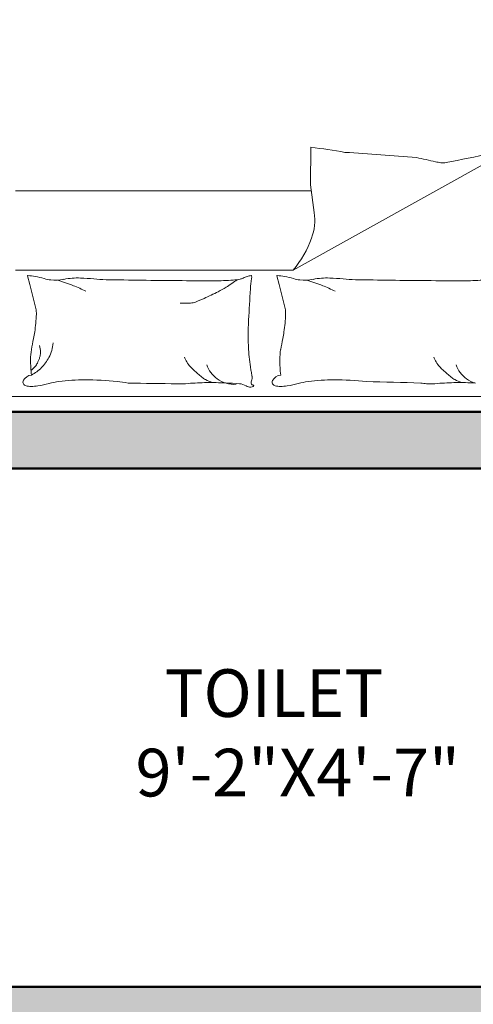
# Model space of a CAD drawing. Units: inches. Extents: x -7 to 1228, y -146 to 1091.
# Tile 72 of 88: x 674 to 722, y 785 to 890. Entities that reach past the tile are written whole.
import ezdxf

# ---------------------------------------------------------------- set-up
doc = ezdxf.new("R2010")
doc.units = ezdxf.units.IN
for name, color, linetype, lineweight in [('A-AREA-IDEN', 7, 'Continuous', 18), ('A-FURN', 8, 'Continuous', 18), ('A-WALL', 7, 'Continuous', 50), ('A-WALL-PATT', 251, 'Continuous', 13)]:
    doc.layers.add(name, color=color, linetype=linetype, lineweight=lineweight)
doc.styles.add('DIM_FONT', font='SIMPLEX.shx', dxfattribs={"width": 0.8})
doc.styles.get("Standard").update_dxf_attribs({"font": 'arial.ttf'})

# ---------------------------------------------------------------- blocks, each defined once
blk = doc.blocks.new('A$C4F634EDD')
for p, q in [((0.5, 2.6295), (2.3, 2.6295)), ((0.5, 2.5771), (2.3, 2.5771)), ((0.5953, 2.1912), (0.616, 2.2738)), ((1.4546, 2.1912), (1.4752, 2.2738)), ((0.5878, 2.1612), (0.5953, 2.1912)), ((1.4471, 2.1612), (1.4546, 2.1912)), ((1.5035, 2.141), (0.5458, 2.141)), ((1.5035, 2.141), (2.2716, 1.7136)), ((1.576, 1.9433), (1.5624, 1.8479)), ((0.5458, 1.8684), (1.5653, 1.8684)), ((1.5624, 1.8479), (1.5641, 1.7178))]:
    blk.add_line(p, q)
for centre, radius, start, end in [((0.5848, 2.5274), 0.0131, 101.2724, 206.5805), ((0.6036, 2.5368), 0.0342, 206.5805, 265.5998), ((0.5999, 2.4516), 0.0904, 90, 101.2724), ((0.5999, 2.3808), 0.1611, 81.5628, 90), ((0.5788, 2.2388), 0.3048, 74.256, 81.5628), ((0.7272, 2.7653), 0.2422, 254.256, 262.4531), ((0.7851, 3.2019), 0.6827, 262.4531, 270), ((0.7851, 3.5682), 1.049, 270, 276.0867), ((0.8402, 3.0514), 0.5293, 276.0867, 280.1899), ((1.1602, -8.1346), 10.6675, 90.30153, 91.21582), ((1.1169, 2.2433), 0.2897, 85.1982, 92.5386), ((1.2142, 3.4021), 0.8732, 265.1982, 269.4243), ((1.2362, 2.45), 0.0768, 117.2396, 128.3886), ((1.3082, 2.3102), 0.234, 110.8603, 117.2396), ((1.2204, 4.0232), 1.4943, 269.4243, 271.9079), ((1.2995, 2.4357), 0.0992, 126.0864, 143.8234), ((1.2995, 2.4357), 0.0992, 105.9352, 126.0864), ((1.2429, 3.3501), 0.8208, 271.9079, 275.2592), ((1.2995, 2.4357), 0.0992, 85.7841, 105.9352), ((1.3132, 2.5864), 0.0539, 275.2592, 300.6513), ((1.3554, 2.5152), 0.0289, 85.6975, 120.6513), ((1.3556, 2.519), 0.0251, 68.2117, 85.6975), ((1.3739, 2.5288), 0.0156, 158.0096, 201.421), ((1.3634, 2.533), 0.00428, 78.1069, 158.0096), ((1.3288, 2.5111), 0.0328, 351.8665, 21.421), ((1.3647, 2.5395), 0.00232, 258.1069, 19.564), ((1.3637, 2.5391), 0.00342, 19.564, 68.2117), ((1.444, 2.5274), 0.0131, 101.2724, 206.5805), ((1.4628, 2.5368), 0.0342, 206.5805, 265.5998), ((1.4591, 2.4516), 0.0904, 90, 101.2724), ((1.4591, 2.3808), 0.1611, 81.5628, 90), ((1.438, 2.2388), 0.3048, 74.256, 81.5628), ((1.5865, 2.7653), 0.2422, 254.256, 262.4531), ((1.6443, 3.2019), 0.6827, 262.4531, 270), ((1.6443, 3.5682), 1.049, 270, 276.0867), ((1.4785, 15.4878), 12.9656, 271.22425, 272.05324), ((1.97, 2.3805), 0.1524, 92.5386, 100.1899), ((1.9761, 2.2433), 0.2897, 85.1982, 92.5386), ((2.0734, 3.4021), 0.8732, 265.1982, 269.4243), ((2.0954, 2.45), 0.0768, 117.2396, 128.3886), ((2.1674, 2.3102), 0.234, 110.8603, 117.2396), ((2.0797, 4.0232), 1.4943, 269.4243, 271.9079), ((2.1588, 2.4357), 0.0992, 126.0864, 143.8234), ((2.1588, 2.4357), 0.0992, 105.9352, 126.0864), ((1.0898, 2.4496), 0.4918, 173.7676, 180), ((0.5462, 2.4142), 0.0899, 41.4429, 53.7359), ((0.5368, 2.3783), 0.1399, 45.0976, 62.7964), ((0.5368, 2.3783), 0.1399, 27.3988, 45.0976), ((1.3165, 2.3233), 0.2252, 133.8115, 140.9651), ((1.4317, 2.2032), 0.3916, 128.3886, 133.8115), ((1.2995, 2.4357), 0.0992, 143.8234, 161.5603), ((1.5522, 2.448), 0.1983, 167.8905, 172.3191), ((1.1177, 2.5413), 0.246, 347.8905, 351.8665), ((1.949, 2.4496), 0.4918, 173.7676, 180), ((2.1757, 2.3233), 0.2252, 133.8115, 140.9651), ((2.291, 2.2032), 0.3916, 128.3886, 133.8115), ((2.1588, 2.4357), 0.0992, 143.8234, 161.5603), ((0.8019, 2.4496), 0.204, 180, 189.6844), ((0.5741, 2.4389), 0.0526, 25.3551, 41.4429), ((0.4851, 2.3967), 0.1511, 21.8149, 25.3551), ((0.4345, 2.3765), 0.2056, 18.7799, 21.8149), ((0.576, 2.4246), 0.0562, 0, 18.7799), ((0.5368, 2.3783), 0.1399, 16.515, 27.3988), ((1.3127, 2.3625), 0.2002, 151.6832, 156.9972), ((1.1799, 2.4341), 0.0493, 140.9651, 151.6832), ((2.2605, 2.3525), 0.9131, 172.3191, 176.6313), ((1.6611, 2.4496), 0.204, 180, 189.6844), ((2.1719, 2.3625), 0.2002, 151.6832, 156.9972), ((2.0391, 2.4341), 0.0493, 140.9651, 151.6832), ((1.4703, 2.5637), 0.882, 189.6844, 192.1984), ((0.5406, 2.4246), 0.0915, 345.3149, 0), ((0.5368, 2.3783), 0.1399, 5.6311, 16.515), ((2.3295, 2.5637), 0.882, 189.6844, 192.1984), ((0.2982, 2.3103), 0.3171, 8.0051, 12.1984), ((2.0266, 2.3663), 0.6787, 176.6313, 181.6331), ((1.1575, 2.3103), 0.3171, 8.0051, 12.1984), ((-0.0401, 2.2627), 0.6588, 2.6649, 8.0051), ((2.7128, 2.3859), 1.3652, 181.6331, 183.055), ((0.8191, 2.2627), 0.6588, 2.6649, 8.0051), ((14.9657, 3.0398), 13.6356, 183.05496, 183.50486), ((0.5503, 2.2902), 0.0677, 345.9548, 2.6649), ((1.4096, 2.2902), 0.0677, 345.9548, 2.6649), ((1.1303, 1.9835), 0.2721, 85.9172, 93.5552), ((1.1455, 2.197), 0.058, 69.3257, 85.9172), ((0.9871, 1.7772), 0.5066, 65.6735, 69.3257), ((0.473, 2.8815), 0.7387, 293.4844, 295.3111), ((0.6058, 0.9338), 1.4323, 63.5015, 65.6735), ((1.1054, 1.9358), 0.3126, 57.865, 63.5015), ((1.6762, 2.2258), 0.3212, 183.5049, 189.9984), ((1.3322, 2.8815), 0.7387, 293.4844, 295.3111), ((0.6807, 2.0561), 0.1197, 96.4341, 107.3864), ((0.6836, 2.0301), 0.1459, 78.4414, 96.4341), ((0.473, 2.8815), 0.7387, 287.1982, 289.428), ((0.759, 2.3985), 0.2301, 258.4414, 272.7491), ((0.473, 2.8815), 0.7387, 289.428, 291.6577), ((0.473, 2.8815), 0.7387, 291.6577, 293.4844), ((0.7026, 3.5718), 1.4048, 272.7491, 274.6176), ((0.9136, 0.9591), 1.2165, 92.6096, 94.6176), ((1.2501, -19.8405), 22.0183, 90.37908, 91.01965), ((1.2012, -3.5404), 5.7185, 89.7135, 90.9704), ((1.224, 1.0141), 1.164, 86.426, 89.7135), ((0.8841, 1.5835), 0.7286, 54.1737, 57.865), ((1.2875, 2.0302), 0.1459, 77.131, 86.426), ((1.3099, 2.1283), 0.0453, 62.7159, 77.131), ((1.5399, 2.0561), 0.1197, 96.4341, 107.3864), ((1.5429, 2.0301), 0.1459, 78.4414, 96.4341), ((1.3322, 2.8815), 0.7387, 287.1982, 289.428), ((1.6182, 2.3985), 0.2301, 258.4414, 272.7491), ((1.3322, 2.8815), 0.7387, 289.428, 291.6577), ((1.3322, 2.8815), 0.7387, 291.6577, 293.4844), ((1.5619, 3.5718), 1.4048, 272.7491, 274.6176), ((1.7729, 0.9591), 1.2165, 92.6096, 94.6176), ((2.1093, -19.8405), 22.0183, 90.37908, 91.01965), ((2.0605, -3.5404), 5.7185, 89.7135, 90.9704), ((2.0833, 1.0141), 1.164, 86.426, 89.7135), ((0.5887, 2.1609), 0.000917, 165.9551, 274.0829), ((0.5695, 2.4301), 0.2708, 274.0829, 279.4841), ((0.5763, 2.3896), 0.2297, 279.4841, 287.3864), ((1.3658, 2.2367), 0.0767, 242.7159, 253.7788), ((1.3688, 2.247), 0.0875, 253.7788, 262.8796), ((1.3581, 2.1615), 0.00132, 262.8796, 343.3022), ((1.3409, 2.1667), 0.0193, 343.3022, 9.9984), ((1.448, 2.1609), 0.000917, 165.9551, 274.0829), ((1.4288, 2.4301), 0.2708, 274.0829, 279.4841), ((1.4355, 2.3896), 0.2297, 279.4841, 287.3864), ((1.2147, 1.9017), 0.3751, 20.1488, 39.6445), ((1.3977, 1.9688), 0.1801, 351.8644, 20.1488), ((1.4194, 4.2174), 2.5158, 281.6741, 283.1904), ((2.0378, 1.5789), 0.1942, 97.7304, 103.1904), ((2.0195, 1.7137), 0.0581, 79.2724, 97.7304), ((1.2737, -2.2227), 4.0646, 77.0745, 79.2724), ((1.0582, 5.4638), 3.7801, 277.692, 279.495), ((0.6102, 18.0525), 16.3521, 273.75703, 274.62393)]:
    blk.add_arc(centre, radius, start, end)
at = {"style": 'DIM_FONT', "width": 0.8, "flags": 9}
for tag, p in [('YSIZE', (0.5, 2.6295)), ('XSIZE', (0.5, 2.6295)), ('XSIZE', (2.2985, 2.6295)), ('YSIZE', (2.2985, 2.6295))]:
    blk.add_attdef(tag, p, '', height=0.0005, dxfattribs=at)

msp = doc.modelspace()

# ---------------------------------------------------------------- hatches: boundary and pattern name
at = {"layer": 'A-WALL-PATT'}
h = msp.add_hatch(color=256, dxfattribs=at)
h.dxf.hatch_style = 1
h.paths.add_polyline_path([(69, 568), (60, 568), (60, 493), (63.29, 493), (69, 493)])
h.paths.add_polyline_path([(69, 662.41), (60, 662.41), (60, 586), (69, 586)], flags=17)
h.paths.add_polyline_path([(69, 723), (184, 723), (184, 734), (179, 734), (179, 728), (69, 728), (69, 741.62), (60, 741.62), (60, 698.41), (69, 698.41)], flags=17)
h.paths.add_polyline_path([(69, 782), (231, 782), (231, 728), (231, 723), (231, 586), (236, 586), (236, 787), (69, 787), (69, 800.13), (60, 800.13), (60, 765.62), (69, 765.62)])
h.paths.add_polyline_path([(184, 842), (189, 842), (189, 848), (173, 848), (173, 842), (179, 842), (179, 787), (184, 787)])
h.paths.add_polyline_path([(118.22, 69), (69, 69), (69, 60), (118.22, 60)])
h.paths.add_polyline_path([(227, 69), (154.22, 69), (154.22, 60), (227, 60)])
h.paths.add_polyline_path([(236, 60), (232.71, 60), (227, 60), (227, 36), (236, 36)])
h.paths.add_polyline_path([(389, 60), (380, 60), (380, 36), (389, 36)])
h.paths.add_polyline_path([(384, 181), (380, 181), (380, 115), (380, 78), (384, 78)])
h.paths.add_polyline_path([(380, 115), (334.55, 115), (334.55, 109), (380, 109)])
h.paths.add_polyline_path([(274.55, 115), (236, 115), (236, 201), (232.71, 201), (231, 201), (231, 78), (236, 78), (236, 109), (274.55, 109)])
h.paths.add_polyline_path([(69, 123), (60, 123), (60, 78), (69, 78)])
h.paths.add_polyline_path([(69, 201), (60, 201), (60, 159), (69, 159)])
h.paths.add_polyline_path([(143, 219), (69, 219), (69, 213), (143, 213)], flags=17)
h.paths.add_polyline_path([(189, 219), (184, 219), (184, 274), (231, 274), (231, 219), (236, 219), (236, 279), (184, 279), (184, 297), (179, 297), (179, 279), (69, 279), (69, 290.91), (60, 290.91), (60, 262.18), (69, 262.18), (69, 274), (179, 274), (179, 219), (173, 219), (173, 213), (189, 213)])
h.paths.add_polyline_path([(69, 238.18), (60, 238.18), (60, 219), (69, 219)], flags=17)
h.paths.add_polyline_path([(69, 333), (60, 333), (60, 314.91), (69, 314.91), (69, 316.96)])
h.paths.add_polyline_path([(190, 338), (184, 338), (69, 338), (69, 333), (179, 333), (179, 327), (184, 327), (184, 333.02), (190, 333.05)])
h.paths.add_polyline_path([(69, 386.81), (60, 386.81), (60, 351), (69, 351)])
h.paths.add_polyline_path([(69, 475), (60, 475), (60, 422.81), (69, 422.81)])
h.paths.add_polyline_path([(236, 475), (231, 475), (231, 351.24), (236, 351.24)])
h.paths.add_polyline_path([(384, 475), (380, 475), (380, 362), (384, 362)])
h.paths.add_polyline_path([(547, 307), (439, 307), (439, 356), (445, 356), (445, 362), (433, 362), (433, 307), (380, 307), (380, 244), (380, 241), (384, 241), (384, 301), (433, 301), (433, 277), (439, 277), (439, 301), (547, 301)])
h.paths.add_polyline_path([(547, 241), (439, 241), (439, 247), (433, 247), (433, 235), (547, 235)])
h.paths.add_polyline_path([(450, 69), (440.29, 69), (424.89, 69), (389, 69), (389, 60), (450, 60)])
h.paths.add_polyline_path([(547, 69), (486, 69), (486, 60), (547, 60)])
h.paths.add_polyline_path([(556, 148.27), (547, 148.27), (547, 78), (556, 78)])
h.paths.add_polyline_path([(556, 223), (547, 223), (547, 195), (547, 184.27), (556, 184.27)])
h.paths.add_polyline_path([(556, 311.19), (547, 311.19), (547, 273.08), (556, 273.08)])
h.paths.add_polyline_path([(556, 344), (552.71, 344), (547, 344), (547, 335.19), (556, 335.19)])
h.paths.add_polyline_path([(556, 249.08), (547, 249.08), (547, 241), (556, 241)])
h.paths.add_polyline_path([(547, 362), (475, 362), (475, 356), (547, 356)], flags=0)
h.paths.add_polyline_path([(556, 399.62), (547, 399.62), (547, 362), (556, 362)])
h.paths.add_polyline_path([(556, 475), (547, 475), (547, 435.62), (556, 435.62)])
h.paths.add_polyline_path([(547, 493), (389, 493), (389, 487), (547, 487)])
h.paths.add_polyline_path([(380, 493), (278, 493), (278, 487), (380, 487)])
h.paths.add_polyline_path([(227, 493), (69, 493), (69, 487), (227, 487)])
h.paths.add_polyline_path([(643, 122.44), (634, 122.44), (634, 78), (643, 78)])
h.paths.add_polyline_path([(702.5, 69), (692.79, 69), (677.39, 69), (643, 69), (643, 60), (702.5, 60)])
h.paths.add_polyline_path([(798, 69), (738.5, 69), (738.5, 60), (798, 60)])
h.paths.add_polyline_path([(807, 60), (803.71, 60), (798, 60), (798, 36), (807, 36)])
h.paths.add_polyline_path([(807, 109), (846.75, 109), (846.75, 115), (807, 115), (807, 159), (802, 159), (802, 78), (807, 78)])
h.paths.add_polyline_path([(807, 201), (802, 201), (802, 195), (807, 195)])
h.paths.add_polyline_path([(643, 201), (634, 201), (634, 158.44), (643, 158.44)])
h.paths.add_polyline_path([(756, 225), (751, 225), (751, 219), (643, 219), (643, 213), (756, 213)])
h.paths.add_polyline_path([(643, 240.85), (634, 240.85), (634, 219), (643, 219)])
h.paths.add_polyline_path([(643, 274), (643, 288.63), (634, 288.63), (634, 264.85), (643, 264.85)])
h.paths.add_polyline_path([(802, 279), (756, 279), (756, 297), (751, 297), (751, 279), (643, 279), (643, 274), (751, 274), (751, 255), (756, 255), (756, 274), (802, 274)])
h.paths.add_polyline_path([(807, 333), (803.71, 333), (802, 333), (802, 279), (802, 274), (802, 219), (807, 219)])
h.paths.add_polyline_path([(956, 182), (951, 182), (951, 115), (906.75, 115), (906.75, 109), (951, 109), (951, 78), (956, 78)])
h.paths.add_polyline_path([(960, 60), (951, 60), (951, 36), (960, 36)])
h.paths.add_polyline_path([(1021, 69), (1005.78, 69), (960, 69), (960, 60), (1021, 60)])
h.paths.add_polyline_path([(956, 224), (951, 224), (951, 218), (956, 218)])
h.paths.add_polyline_path([(956, 302), (1004, 302), (1004, 278), (1010, 278), (1010, 302), (1118, 302), (1118, 290.81), (1127, 290.81), (1127, 326.97), (1118, 326.97), (1118, 320.97), (1118, 307), (1010, 307), (1010, 356), (1016, 356), (1016, 362), (1004, 362), (1004, 307), (951, 307), (951, 244), (951, 242), (954.29, 242), (956, 242)])
h.paths.add_polyline_path([(643, 333), (634, 333), (634, 312.63), (643, 312.63), (643, 316.96)])
h.paths.add_polyline_path([(756, 338), (643, 338), (643, 333), (751, 333), (751, 327), (756, 327)])
h.paths.add_polyline_path([(643, 388), (634, 388), (634, 351), (643, 351)])
h.paths.add_polyline_path([(807, 357), (802, 357), (802, 351), (807, 351)])
h.paths.add_polyline_path([(807, 475), (802, 475), (802, 393), (807, 393)])
h.paths.add_polyline_path([(643, 475), (634, 475), (634, 424), (643, 424)])
h.paths.add_polyline_path([(798, 493), (643, 493), (643, 487), (798, 487)])
h.paths.add_polyline_path([(634, 493), (556, 493), (556, 487), (634, 487)])
h.paths.add_polyline_path([(813, 493), (807, 493), (807, 487), (813, 487)])
h.paths.add_polyline_path([(951, 493), (849, 493), (849, 487), (951, 487)])
h.paths.add_polyline_path([(956, 484), (951, 484), (951, 374), (956, 374)])
h.paths.add_polyline_path([(1109, 493), (969, 493), (969, 487), (1109, 487)])
h.paths.add_polyline_path([(1127, 484), (1118, 484), (1118, 450.64), (1127, 450.64)])
h.paths.add_polyline_path([(1127, 414.64), (1118, 414.64), (1118, 365), (1127, 365)])
h.paths.add_polyline_path([(1109, 362), (1046, 362), (1046, 356), (1109, 356)], flags=17)
h.paths.add_polyline_path([(1127, 356), (1123.45, 356), (1118, 356), (1118, 350.97), (1127, 350.97)], flags=0)
h.paths.add_polyline_path([(1127, 266.81), (1118, 266.81), (1118, 262.36), (1118, 242), (1127, 242)], flags=17)
h.paths.add_polyline_path([(1118, 242), (1010, 242), (1010, 248), (1004, 248), (1004, 237), (1118, 237)])
h.paths.add_polyline_path([(1127, 224), (1118, 224), (1118, 170), (1127, 170)])
h.paths.add_polyline_path([(1127, 134), (1118, 134), (1118, 78), (1127, 78)])
h.paths.add_polyline_path([(1118, 69), (1057, 69), (1057, 60), (1118, 60)])
h.paths.add_polyline_path([(227, 571.55), (227, 574), (69, 574), (69, 568), (227, 568)])
h.paths.add_polyline_path([(380, 571.55), (380, 574), (278, 574), (278, 568), (380, 568)])
h.paths.add_polyline_path([(242, 574), (236, 574), (236, 568), (242, 568)])
h.paths.add_polyline_path([(547, 571.55), (547, 574), (389, 574), (389, 568), (547, 568)])
h.paths.add_polyline_path([(384, 733), (380, 733), (380, 586), (384, 586)])
h.paths.add_polyline_path([(556, 646), (634, 646), (634, 655), (547, 655), (547, 586), (556, 586)])
h.paths.add_polyline_path([(634, 574), (556, 574), (556, 568), (634, 568)])
h.paths.add_polyline_path([(643, 655), (634, 655), (634, 586), (643, 586)])
h.paths.add_polyline_path([(798, 574), (643, 574), (643, 568), (798, 568)])
h.paths.add_polyline_path([(643, 663.85), (634, 663.85), (634, 655), (643, 655)])
h.paths.add_polyline_path([(556, 676.97), (547, 676.97), (547, 655), (556, 655)])
h.paths.add_polyline_path([(556, 733), (547, 733), (547, 712.97), (556, 712.97)])
h.paths.add_polyline_path([(643, 710), (634, 710), (634, 699.85), (643, 699.85)])
h.paths.add_polyline_path([(807, 668), (802, 668), (802, 586), (807, 586)])
h.paths.add_polyline_path([(951, 574), (849, 574), (849, 568), (951, 568)])
h.paths.add_polyline_path([(956, 691), (951, 691), (951, 577), (956, 577)])
h.paths.add_polyline_path([(1109, 574), (969, 574), (969, 568), (1109, 568)])
h.paths.add_polyline_path([(1127, 643.4), (1118, 643.4), (1118, 577), (1127, 577)])
h.paths.add_polyline_path([(1127, 568), (1123.45, 568), (1118, 568), (1118, 493), (1127, 493)])
h.paths.add_polyline_path([(1127, 733), (1118, 733), (1118, 679.4), (1127, 679.4)])
h.paths.add_polyline_path([(1127, 777.35), (1118, 777.35), (1118, 770.04), (1118, 751), (1127, 751)], flags=17)
h.paths.add_polyline_path([(1118, 751), (1010, 751), (1010, 757), (1004, 757), (1004, 745), (1118, 745)])
h.paths.add_polyline_path([(956, 811), (1004, 811), (1004, 787), (1010, 787), (1010, 811), (1017.87, 811), (1017.87, 811.63, -0.414214), (1018.25, 812), (1031.98, 812, -0.414214), (1032.35, 811.63), (1032.35, 811), (1118, 811), (1118, 801.35), (1127, 801.35), (1127, 834.69), (1118, 834.69), (1118, 830.24), (1118, 817), (1010, 817), (1010, 866), (1016, 866), (1016, 872), (1004, 872), (1004, 817), (956, 817), (956, 866), (951, 866), (951, 751), (954.29, 751), (956, 751)])
h.paths.add_polyline_path([(1118, 872), (1046, 872), (1046, 866), (1118, 866)], flags=17)
h.paths.add_polyline_path([(1127, 924.71), (1118, 924.71), (1118, 884), (1127, 884)])
h.paths.add_polyline_path([(1127, 866), (1123.71, 866), (1118, 866), (1118, 858.69), (1127, 858.69)], flags=17)
h.paths.add_polyline_path([(956, 983), (951, 983), (951, 952), (807, 952), (807, 983), (802, 983), (802, 902), (807, 902), (807, 946), (951, 946), (951, 884), (956, 884)])
h.paths.add_polyline_path([(807, 842), (802, 842), (802, 787), (756, 787), (756, 806), (751, 806), (751, 787), (643, 787), (643, 782), (751, 782), (751, 764), (756, 764), (756, 782), (802, 782), (802, 728), (807, 728)])
h.paths.add_polyline_path([(756, 848), (643, 848), (643, 842), (751, 842), (751, 836), (756, 836)])
h.paths.add_polyline_path([(756, 734), (751, 734), (751, 728), (643, 728), (643, 723), (756, 723)])
h.paths.add_polyline_path([(643, 749.79), (634, 749.79), (634, 728), (637.29, 728), (643, 728)])
h.paths.add_polyline_path([(643, 805.41), (634, 805.41), (634, 773.79), (643, 773.79)])
h.paths.add_polyline_path([(643, 896.66), (634, 896.66), (634, 860), (637.29, 860), (643, 860)])
h.paths.add_polyline_path([(643, 842), (634, 842), (634, 829.41), (643, 829.41)])
h.paths.add_polyline_path([(643, 983), (634, 983), (634, 932.66), (643, 932.66)])
h.paths.add_polyline_path([(1127, 983), (1118, 983), (1118, 960.71), (1127, 960.71)])
h.paths.add_polyline_path([(1118, 1001), (1077.53, 1001), (1077.53, 992), (1118, 992)])
h.paths.add_polyline_path([(1041.53, 1001), (960, 1001), (960, 992), (1041.53, 992)])
h.paths.add_polyline_path([(960, 1025), (951, 1025), (951, 1001), (954.29, 1001), (960, 1001)])
h.paths.add_polyline_path([(807, 1025), (798, 1025), (798, 1001), (807, 1001)])
h.paths.add_polyline_path([(798, 1001), (738.5, 1001), (738.5, 992), (798, 992)])
h.paths.add_polyline_path([(702.5, 1001), (643, 1001), (643, 992), (702.5, 992)])
h.paths.add_polyline_path([(547, 1001), (499.11, 1001), (499.11, 992), (547, 992)])
h.paths.add_polyline_path([(463.11, 1001), (389, 1001), (389, 992), (463.11, 992)])
h.paths.add_polyline_path([(389, 1025), (380, 1025), (380, 1022), (380, 1001), (383.29, 1001), (389, 1001)])
h.paths.add_polyline_path([(236, 1025), (227, 1025), (227, 1001), (236, 1001)])
h.paths.add_polyline_path([(236, 983), (231, 983), (231, 860), (236, 860)])
h.paths.add_polyline_path([(274.55, 952), (236, 952), (236, 946), (274.55, 946)])
h.paths.add_polyline_path([(380, 952), (334.55, 952), (334.55, 946), (380, 946)])
h.paths.add_polyline_path([(384, 983), (380, 983), (380, 884), (383.29, 884), (384, 884)])
h.paths.add_polyline_path([(227, 1001), (155.01, 1001), (155.01, 992), (162.87, 992), (227, 992)])
h.paths.add_polyline_path([(119.01, 1001), (69, 1001), (69, 992), (119.01, 992)])
h.paths.add_polyline_path([(69, 983), (60, 983), (60, 922.99), (69, 922.99)])
h.paths.add_polyline_path([(69, 886.99), (60, 886.99), (60, 860), (63.29, 860), (69, 860)])
h.paths.add_polyline_path([(143, 848), (69, 848), (69, 842), (143, 842)])

# ---------------------------------------------------------------- linework, layer by layer
at = {"layer": 'A-WALL'}
for p, q in [((756, 848), (643, 848)), ((751, 842), (643, 842)), ((751, 787), (643, 787))]:
    msp.add_line(p, q, dxfattribs=at)

# ---------------------------------------------------------------- block references
at = {"layer": 'A-FURN', "xscale": -30.79356024027943, "yscale": 30.79356024027943, "zscale": 30.79356024027943, "rotation": 180}
msp.add_blockref('A$C4F634EDD', (656.39, 928.97), dxfattribs=at)

# ---------------------------------------------------------------- texts
at = {"layer": 'A-AREA-IDEN', "insert": (685.94, 820.68), "char_height": 5.0568, "attachment_point": 1}
msp.add_mtext_dynamic_manual_height_columns('  TOILET\\P9\'-2"X4\'-7"', width=137.2821, gutter_width=25.28, heights=[0], dxfattribs=at)

doc.saveas('drawing.dxf')
